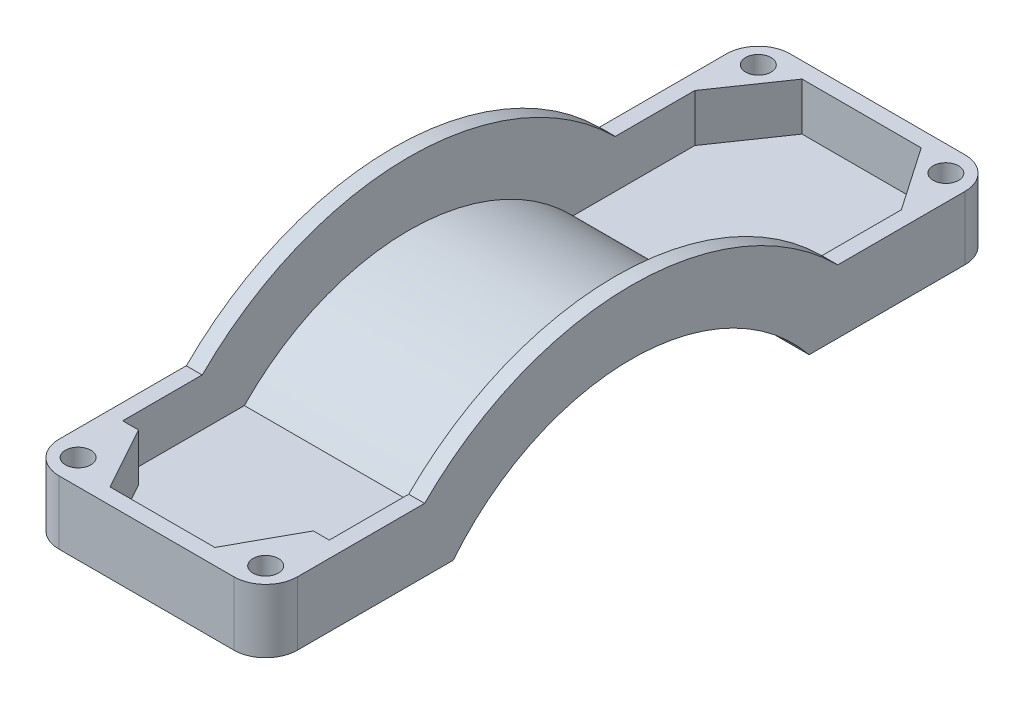
ISO-10303-21;
HEADER;
FILE_DESCRIPTION(('STEP AP214'),'2;1');
FILE_NAME('part.step','',(''),(''),'','','');
FILE_SCHEMA(('AUTOMOTIVE_DESIGN { 1 0 10303 214 1 1 1 1 }'));
ENDSEC;
DATA;
#1=APPLICATION_CONTEXT('core data for automotive mechanical design processes');
#2=APPLICATION_PROTOCOL_DEFINITION('international standard','automotive_design',2000,#1);
#3=PRODUCT_CONTEXT('',#1,'mechanical');
#4=PRODUCT('Part','Part','',(#3));
#5=PRODUCT_RELATED_PRODUCT_CATEGORY('part','',(#4));
#6=PRODUCT_DEFINITION_FORMATION('','',#4);
#7=PRODUCT_DEFINITION_CONTEXT('part definition',#1,'design');
#8=PRODUCT_DEFINITION('design','',#6,#7);
#9=PRODUCT_DEFINITION_SHAPE('','',#8);
#10=(LENGTH_UNIT() NAMED_UNIT(*) SI_UNIT(.MILLI.,.METRE.));
#11=(NAMED_UNIT(*) PLANE_ANGLE_UNIT() SI_UNIT($,.RADIAN.));
#12=(NAMED_UNIT(*) SI_UNIT($,.STERADIAN.) SOLID_ANGLE_UNIT());
#13=UNCERTAINTY_MEASURE_WITH_UNIT(LENGTH_MEASURE(1.E-05),#10,'distance_accuracy_value','');
#14=(GEOMETRIC_REPRESENTATION_CONTEXT(3) GLOBAL_UNCERTAINTY_ASSIGNED_CONTEXT((#13)) GLOBAL_UNIT_ASSIGNED_CONTEXT((#10,
#11,#12)) REPRESENTATION_CONTEXT('',''));
#15=CARTESIAN_POINT('',(0.,0.,0.));
#16=DIRECTION('',(0.,0.,1.));
#17=DIRECTION('',(1.,0.,0.));
#18=AXIS2_PLACEMENT_3D('',#15,#16,#17);
#19=CARTESIAN_POINT('',(-5.,0.,0.));
#20=DIRECTION('',(1.,0.,0.));
#21=DIRECTION('',(0.,0.,-1.));
#22=AXIS2_PLACEMENT_3D('',#19,#20,#21);
#23=PLANE('',#22);
#24=DIRECTION('',(0.,0.,-1.));
#25=VECTOR('',#24,1.);
#26=CARTESIAN_POINT('',(-5.00000000000001,50.1076032426321,0.));
#27=LINE('',#26,#25);
#28=CARTESIAN_POINT('',(-5.,50.1076032426321,-51.7032696962094));
#29=VERTEX_POINT('',#28);
#30=CARTESIAN_POINT('',(-5.,50.1076032426321,-90.));
#31=VERTEX_POINT('',#30);
#32=EDGE_CURVE('E569',#29,#31,#27,.T.);
#33=ORIENTED_EDGE('',*,*,#32,.F.);
#34=CARTESIAN_POINT('',(-5.,0.,0.));
#35=DIRECTION('',(1.,0.,0.));
#36=DIRECTION('',(0.,0.,-1.));
#37=AXIS2_PLACEMENT_3D('',#34,#35,#36);
#38=CIRCLE('',#37,72.);
#39=CARTESIAN_POINT('',(-5.,50.1076032426321,51.7032696962094));
#40=VERTEX_POINT('',#39);
#41=EDGE_CURVE('E249',#29,#40,#38,.T.);
#42=ORIENTED_EDGE('',*,*,#41,.T.);
#43=DIRECTION('',(0.,0.,1.));
#44=VECTOR('',#43,1.);
#45=CARTESIAN_POINT('',(-4.99999999999999,50.1076032426321,0.));
#46=LINE('',#45,#44);
#47=CARTESIAN_POINT('',(-5.,50.1076032426321,90.));
#48=VERTEX_POINT('',#47);
#49=EDGE_CURVE('E296',#40,#48,#46,.T.);
#50=ORIENTED_EDGE('',*,*,#49,.T.);
#51=DIRECTION('',(0.,1.,0.));
#52=VECTOR('',#51,1.);
#53=CARTESIAN_POINT('',(-5.,50.1076032426321,90.));
#54=LINE('',#53,#52);
#55=CARTESIAN_POINT('',(-5.,65.1076032426321,90.));
#56=VERTEX_POINT('',#55);
#57=EDGE_CURVE('E333',#48,#56,#54,.T.);
#58=ORIENTED_EDGE('',*,*,#57,.T.);
#59=DIRECTION('',(0.,0.,1.));
#60=VECTOR('',#59,1.);
#61=CARTESIAN_POINT('',(-4.99999999999999,65.1076032426321,0.));
#62=LINE('',#61,#60);
#63=CARTESIAN_POINT('',(-5.,65.1076032426321,65.));
#64=VERTEX_POINT('',#63);
#65=EDGE_CURVE('E317',#64,#56,#62,.T.);
#66=ORIENTED_EDGE('',*,*,#65,.F.);
#67=CARTESIAN_POINT('',(-5.,0.,0.));
#68=DIRECTION('',(1.,0.,0.));
#69=DIRECTION('',(0.,0.,-1.));
#70=AXIS2_PLACEMENT_3D('',#67,#68,#69);
#71=CIRCLE('',#70,92.);
#72=CARTESIAN_POINT('',(-5.,65.1076032426321,-65.));
#73=VERTEX_POINT('',#72);
#74=EDGE_CURVE('E348',#73,#64,#71,.T.);
#75=ORIENTED_EDGE('',*,*,#74,.F.);
#76=DIRECTION('',(0.,0.,-1.));
#77=VECTOR('',#76,1.);
#78=CARTESIAN_POINT('',(-5.00000000000001,65.1076032426321,0.));
#79=LINE('',#78,#77);
#80=CARTESIAN_POINT('',(-5.,65.1076032426321,-90.));
#81=VERTEX_POINT('',#80);
#82=EDGE_CURVE('E252',#73,#81,#79,.T.);
#83=ORIENTED_EDGE('',*,*,#82,.T.);
#84=DIRECTION('',(0.,1.,0.));
#85=VECTOR('',#84,1.);
#86=CARTESIAN_POINT('',(-5.,50.1076032426321,-90.));
#87=LINE('',#86,#85);
#88=EDGE_CURVE('E243',#31,#81,#87,.T.);
#89=ORIENTED_EDGE('',*,*,#88,.F.);
#90=EDGE_LOOP('',(#33,#42,#50,#58,#66,#75,#83,#89));
#91=FACE_BOUND('',#90,.T.);
#92=ADVANCED_FACE('F50',(#91),#23,.F.);
#93=CARTESIAN_POINT('',(-70.,50.1076032426321,0.));
#94=DIRECTION('',(1.,0.,0.));
#95=DIRECTION('',(0.,0.,-1.));
#96=AXIS2_PLACEMENT_3D('',#93,#94,#95);
#97=PLANE('',#96);
#98=CARTESIAN_POINT('',(-70.,0.,0.));
#99=DIRECTION('',(-1.,0.,0.));
#100=DIRECTION('',(0.,0.,1.));
#101=AXIS2_PLACEMENT_3D('',#98,#99,#100);
#102=CIRCLE('',#101,72.);
#103=CARTESIAN_POINT('',(-70.,50.1076032426321,51.7032696962094));
#104=VERTEX_POINT('',#103);
#105=CARTESIAN_POINT('',(-70.,50.1076032426321,-51.7032696962094));
#106=VERTEX_POINT('',#105);
#107=EDGE_CURVE('E248',#104,#106,#102,.T.);
#108=ORIENTED_EDGE('',*,*,#107,.T.);
#109=DIRECTION('',(0.,0.,1.));
#110=VECTOR('',#109,1.);
#111=CARTESIAN_POINT('',(-70.,50.1076032426321,0.));
#112=LINE('',#111,#110);
#113=CARTESIAN_POINT('',(-70.,50.1076032426321,-90.));
#114=VERTEX_POINT('',#113);
#115=EDGE_CURVE('E231',#114,#106,#112,.T.);
#116=ORIENTED_EDGE('',*,*,#115,.F.);
#117=DIRECTION('',(0.,1.,0.));
#118=VECTOR('',#117,1.);
#119=CARTESIAN_POINT('',(-70.,50.1076032426321,-90.));
#120=LINE('',#119,#118);
#121=CARTESIAN_POINT('',(-70.,65.1076032426321,-90.));
#122=VERTEX_POINT('',#121);
#123=EDGE_CURVE('E561',#114,#122,#120,.T.);
#124=ORIENTED_EDGE('',*,*,#123,.T.);
#125=DIRECTION('',(0.,0.,1.));
#126=VECTOR('',#125,1.);
#127=CARTESIAN_POINT('',(-70.,65.1076032426321,0.));
#128=LINE('',#127,#126);
#129=CARTESIAN_POINT('',(-70.,65.1076032426321,-65.));
#130=VERTEX_POINT('',#129);
#131=EDGE_CURVE('E568',#122,#130,#128,.T.);
#132=ORIENTED_EDGE('',*,*,#131,.T.);
#133=DIRECTION('',(0.,1.,0.));
#134=VECTOR('',#133,1.);
#135=CARTESIAN_POINT('',(-70.,0.,-65.));
#136=LINE('',#135,#134);
#137=CARTESIAN_POINT('',(-70.,65.0438347815245,-65.));
#138=VERTEX_POINT('',#137);
#139=EDGE_CURVE('E379',#138,#130,#136,.T.);
#140=ORIENTED_EDGE('',*,*,#139,.F.);
#141=CARTESIAN_POINT('',(-70.,0.,0.));
#142=DIRECTION('',(-1.,0.,0.));
#143=DIRECTION('',(0.,0.,1.));
#144=AXIS2_PLACEMENT_3D('',#141,#142,#143);
#145=CIRCLE('',#144,91.954882649516);
#146=CARTESIAN_POINT('',(-70.,65.0438347815245,65.));
#147=VERTEX_POINT('',#146);
#148=EDGE_CURVE('E257',#147,#138,#145,.T.);
#149=ORIENTED_EDGE('',*,*,#148,.F.);
#150=DIRECTION('',(0.,1.,0.));
#151=VECTOR('',#150,1.);
#152=CARTESIAN_POINT('',(-70.,50.1076032426321,65.));
#153=LINE('',#152,#151);
#154=CARTESIAN_POINT('',(-70.,65.1076032426321,65.));
#155=VERTEX_POINT('',#154);
#156=EDGE_CURVE('E326',#147,#155,#153,.T.);
#157=ORIENTED_EDGE('',*,*,#156,.T.);
#158=DIRECTION('',(0.,0.,-1.));
#159=VECTOR('',#158,1.);
#160=CARTESIAN_POINT('',(-70.,65.1076032426321,0.));
#161=LINE('',#160,#159);
#162=CARTESIAN_POINT('',(-70.,65.1076032426321,90.));
#163=VERTEX_POINT('',#162);
#164=EDGE_CURVE('E316',#163,#155,#161,.T.);
#165=ORIENTED_EDGE('',*,*,#164,.F.);
#166=DIRECTION('',(0.,1.,0.));
#167=VECTOR('',#166,1.);
#168=CARTESIAN_POINT('',(-70.,50.1076032426321,90.));
#169=LINE('',#168,#167);
#170=CARTESIAN_POINT('',(-70.,50.1076032426321,90.));
#171=VERTEX_POINT('',#170);
#172=EDGE_CURVE('E329',#171,#163,#169,.T.);
#173=ORIENTED_EDGE('',*,*,#172,.F.);
#174=DIRECTION('',(0.,0.,-1.));
#175=VECTOR('',#174,1.);
#176=CARTESIAN_POINT('',(-70.,50.1076032426321,0.));
#177=LINE('',#176,#175);
#178=EDGE_CURVE('E256',#171,#104,#177,.T.);
#179=ORIENTED_EDGE('',*,*,#178,.T.);
#180=EDGE_LOOP('',(#108,#116,#124,#132,#140,#149,#157,#165,#173,#179));
#181=FACE_BOUND('',#180,.T.);
#182=ADVANCED_FACE('F251',(#181),#97,.T.);
#183=CARTESIAN_POINT('',(-70.,0.,0.));
#184=DIRECTION('',(-1.,0.,0.));
#185=DIRECTION('',(0.,0.,1.));
#186=AXIS2_PLACEMENT_3D('',#183,#184,#185);
#187=CYLINDRICAL_SURFACE('',#186,91.954882649516);
#188=ORIENTED_EDGE('',*,*,#148,.T.);
#189=DIRECTION('',(-1.,0.,0.));
#190=VECTOR('',#189,1.);
#191=CARTESIAN_POINT('',(-70.,65.0438347815245,-65.));
#192=LINE('',#191,#190);
#193=CARTESIAN_POINT('',(-75.,65.0438347815245,-65.));
#194=VERTEX_POINT('',#193);
#195=EDGE_CURVE('E370',#138,#194,#192,.T.);
#196=ORIENTED_EDGE('',*,*,#195,.T.);
#197=CARTESIAN_POINT('',(-75.,0.,0.));
#198=DIRECTION('',(-1.,0.,0.));
#199=DIRECTION('',(0.,0.,1.));
#200=AXIS2_PLACEMENT_3D('',#197,#198,#199);
#201=CIRCLE('',#200,91.954882649516);
#202=CARTESIAN_POINT('',(-75.,65.0438347815245,65.));
#203=VERTEX_POINT('',#202);
#204=EDGE_CURVE('E258',#203,#194,#201,.T.);
#205=ORIENTED_EDGE('',*,*,#204,.F.);
#206=DIRECTION('',(-1.,0.,0.));
#207=VECTOR('',#206,1.);
#208=CARTESIAN_POINT('',(-70.,65.0438347815245,65.));
#209=LINE('',#208,#207);
#210=EDGE_CURVE('E264',#147,#203,#209,.T.);
#211=ORIENTED_EDGE('',*,*,#210,.F.);
#212=EDGE_LOOP('',(#188,#196,#205,#211));
#213=FACE_BOUND('',#212,.T.);
#214=ADVANCED_FACE('F459',(#213),#187,.T.);
#215=CARTESIAN_POINT('',(-75.,0.,0.));
#216=DIRECTION('',(1.,0.,0.));
#217=DIRECTION('',(0.,0.,-1.));
#218=AXIS2_PLACEMENT_3D('',#215,#216,#217);
#219=CYLINDRICAL_SURFACE('',#218,72.);
#220=DIRECTION('',(1.,0.,0.));
#221=VECTOR('',#220,1.);
#222=CARTESIAN_POINT('',(-75.,50.1076032426321,-51.7032696962094));
#223=LINE('',#222,#221);
#224=EDGE_CURVE('E240',#106,#29,#223,.T.);
#225=ORIENTED_EDGE('',*,*,#224,.F.);
#226=ORIENTED_EDGE('',*,*,#107,.F.);
#227=DIRECTION('',(1.,0.,0.));
#228=VECTOR('',#227,1.);
#229=CARTESIAN_POINT('',(-75.,50.1076032426321,51.7032696962094));
#230=LINE('',#229,#228);
#231=EDGE_CURVE('E263',#40,#104,#230,.F.);
#232=ORIENTED_EDGE('',*,*,#231,.F.);
#233=ORIENTED_EDGE('',*,*,#41,.F.);
#234=EDGE_LOOP('',(#225,#226,#232,#233));
#235=FACE_BOUND('',#234,.T.);
#236=ADVANCED_FACE('F250',(#235),#219,.T.);
#237=CARTESIAN_POINT('',(-5.,65.1076032426321,0.));
#238=DIRECTION('',(0.,1.,0.));
#239=DIRECTION('',(0.,0.,1.));
#240=AXIS2_PLACEMENT_3D('',#237,#238,#239);
#241=PLANE('',#240);
#242=CARTESIAN_POINT('',(-8.,65.1076032426321,107.));
#243=DIRECTION('',(0.,1.,0.));
#244=DIRECTION('',(0.,0.,1.));
#245=AXIS2_PLACEMENT_3D('',#242,#243,#244);
#246=CIRCLE('',#245,4.);
#247=CARTESIAN_POINT('',(-8.,65.1076032426321,111.));
#248=VERTEX_POINT('',#247);
#249=EDGE_CURVE('E593',#248,#248,#246,.T.);
#250=ORIENTED_EDGE('',*,*,#249,.F.);
#251=EDGE_LOOP('',(#250));
#252=FACE_BOUND('',#251,.T.);
#253=CARTESIAN_POINT('',(-67.,65.1076032426321,107.));
#254=DIRECTION('',(0.,1.,0.));
#255=DIRECTION('',(0.,0.,1.));
#256=AXIS2_PLACEMENT_3D('',#253,#254,#255);
#257=CIRCLE('',#256,4.00000000000001);
#258=CARTESIAN_POINT('',(-67.,65.1076032426321,111.));
#259=VERTEX_POINT('',#258);
#260=EDGE_CURVE('E595',#259,#259,#257,.T.);
#261=ORIENTED_EDGE('',*,*,#260,.F.);
#262=EDGE_LOOP('',(#261));
#263=FACE_BOUND('',#262,.T.);
#264=DIRECTION('',(0.,0.,1.));
#265=VECTOR('',#264,1.);
#266=CARTESIAN_POINT('',(-75.,65.1076032426321,65.));
#267=LINE('',#266,#265);
#268=CARTESIAN_POINT('',(-75.,65.1076032426321,65.));
#269=VERTEX_POINT('',#268);
#270=CARTESIAN_POINT('',(-75.,65.1076032426321,105.));
#271=VERTEX_POINT('',#270);
#272=EDGE_CURVE('E345',#269,#271,#267,.T.);
#273=ORIENTED_EDGE('',*,*,#272,.T.);
#274=CARTESIAN_POINT('',(-65.,65.1076032426321,105.));
#275=DIRECTION('',(0.,1.,0.));
#276=DIRECTION('',(0.,0.,1.));
#277=AXIS2_PLACEMENT_3D('',#274,#275,#276);
#278=CIRCLE('',#277,10.);
#279=CARTESIAN_POINT('',(-65.,65.1076032426321,115.));
#280=VERTEX_POINT('',#279);
#281=EDGE_CURVE('E415',#271,#280,#278,.T.);
#282=ORIENTED_EDGE('',*,*,#281,.T.);
#283=DIRECTION('',(1.,0.,0.));
#284=VECTOR('',#283,1.);
#285=CARTESIAN_POINT('',(-5.,65.1076032426321,115.));
#286=LINE('',#285,#284);
#287=CARTESIAN_POINT('',(-10.,65.1076032426321,115.));
#288=VERTEX_POINT('',#287);
#289=EDGE_CURVE('E368',#280,#288,#286,.T.);
#290=ORIENTED_EDGE('',*,*,#289,.T.);
#291=CARTESIAN_POINT('',(-10.,65.1076032426321,105.));
#292=DIRECTION('',(0.,1.,0.));
#293=DIRECTION('',(0.,0.,1.));
#294=AXIS2_PLACEMENT_3D('',#291,#292,#293);
#295=CIRCLE('',#294,10.);
#296=CARTESIAN_POINT('',(0.,65.1076032426321,105.));
#297=VERTEX_POINT('',#296);
#298=EDGE_CURVE('E404',#288,#297,#295,.T.);
#299=ORIENTED_EDGE('',*,*,#298,.T.);
#300=DIRECTION('',(0.,0.,1.));
#301=VECTOR('',#300,1.);
#302=CARTESIAN_POINT('',(0.,65.1076032426321,0.));
#303=LINE('',#302,#301);
#304=CARTESIAN_POINT('',(0.,65.1076032426321,65.));
#305=VERTEX_POINT('',#304);
#306=EDGE_CURVE('E363',#305,#297,#303,.T.);
#307=ORIENTED_EDGE('',*,*,#306,.F.);
#308=DIRECTION('',(1.,0.,0.));
#309=VECTOR('',#308,1.);
#310=CARTESIAN_POINT('',(-5.,65.1076032426321,65.));
#311=LINE('',#310,#309);
#312=EDGE_CURVE('E369',#64,#305,#311,.T.);
#313=ORIENTED_EDGE('',*,*,#312,.F.);
#314=ORIENTED_EDGE('',*,*,#65,.T.);
#315=DIRECTION('',(-1.,0.,0.));
#316=VECTOR('',#315,1.);
#317=CARTESIAN_POINT('',(0.,65.1076032426321,90.));
#318=LINE('',#317,#316);
#319=CARTESIAN_POINT('',(-10.,65.1076032426321,90.));
#320=VERTEX_POINT('',#319);
#321=EDGE_CURVE('E312',#56,#320,#318,.T.);
#322=ORIENTED_EDGE('',*,*,#321,.T.);
#323=DIRECTION('',(0.481918749772156,0.,-0.876215908676647));
#324=VECTOR('',#323,1.);
#325=CARTESIAN_POINT('',(30.3262955854127,65.1076032426321,16.679462571977));
#326=LINE('',#325,#324);
#327=CARTESIAN_POINT('',(-21.,65.1076032426321,110.));
#328=VERTEX_POINT('',#327);
#329=EDGE_CURVE('E309',#328,#320,#326,.T.);
#330=ORIENTED_EDGE('',*,*,#329,.F.);
#331=DIRECTION('',(1.,0.,0.));
#332=VECTOR('',#331,1.);
#333=CARTESIAN_POINT('',(0.,65.1076032426321,110.));
#334=LINE('',#333,#332);
#335=CARTESIAN_POINT('',(-54.,65.1076032426321,110.));
#336=VERTEX_POINT('',#335);
#337=EDGE_CURVE('E310',#336,#328,#334,.T.);
#338=ORIENTED_EDGE('',*,*,#337,.F.);
#339=DIRECTION('',(0.481918749772156,0.,0.876215908676647));
#340=VECTOR('',#339,1.);
#341=CARTESIAN_POINT('',(-87.9078694817658,65.1076032426321,48.3493282149712));
#342=LINE('',#341,#340);
#343=CARTESIAN_POINT('',(-65.,65.1076032426321,90.));
#344=VERTEX_POINT('',#343);
#345=EDGE_CURVE('E285',#344,#336,#342,.T.);
#346=ORIENTED_EDGE('',*,*,#345,.F.);
#347=DIRECTION('',(1.,0.,0.));
#348=VECTOR('',#347,1.);
#349=CARTESIAN_POINT('',(0.,65.1076032426321,90.));
#350=LINE('',#349,#348);
#351=EDGE_CURVE('E286',#163,#344,#350,.T.);
#352=ORIENTED_EDGE('',*,*,#351,.F.);
#353=ORIENTED_EDGE('',*,*,#164,.T.);
#354=DIRECTION('',(-1.,0.,0.));
#355=VECTOR('',#354,1.);
#356=CARTESIAN_POINT('',(-5.,65.1076032426321,65.));
#357=LINE('',#356,#355);
#358=EDGE_CURVE('E327',#155,#269,#357,.T.);
#359=ORIENTED_EDGE('',*,*,#358,.T.);
#360=EDGE_LOOP('',(#273,#282,#290,#299,#307,#313,#314,#322,#330,#338,#346,#352,#353,#359));
#361=FACE_BOUND('',#360,.T.);
#362=ADVANCED_FACE('F477',(#252,#263,#361),#241,.T.);
#363=CARTESIAN_POINT('',(0.,0.,65.));
#364=DIRECTION('',(0.,0.,-1.));
#365=DIRECTION('',(-1.,0.,0.));
#366=AXIS2_PLACEMENT_3D('',#363,#364,#365);
#367=PLANE('',#366);
#368=ORIENTED_EDGE('',*,*,#210,.T.);
#369=DIRECTION('',(0.,-1.,0.));
#370=VECTOR('',#369,1.);
#371=CARTESIAN_POINT('',(-75.,45.1076032426321,65.));
#372=LINE('',#371,#370);
#373=EDGE_CURVE('E339',#269,#203,#372,.T.);
#374=ORIENTED_EDGE('',*,*,#373,.F.);
#375=ORIENTED_EDGE('',*,*,#358,.F.);
#376=ORIENTED_EDGE('',*,*,#156,.F.);
#377=EDGE_LOOP('',(#368,#374,#375,#376));
#378=FACE_BOUND('',#377,.T.);
#379=ADVANCED_FACE('F468',(#378),#367,.T.);
#380=CARTESIAN_POINT('',(-5.,45.1076032426321,0.));
#381=DIRECTION('',(0.,-1.,0.));
#382=DIRECTION('',(0.,0.,-1.));
#383=AXIS2_PLACEMENT_3D('',#380,#381,#382);
#384=PLANE('',#383);
#385=CARTESIAN_POINT('',(-8.,45.1076032426321,107.));
#386=DIRECTION('',(0.,-1.,0.));
#387=DIRECTION('',(0.,0.,-1.));
#388=AXIS2_PLACEMENT_3D('',#385,#386,#387);
#389=CIRCLE('',#388,4.);
#390=CARTESIAN_POINT('',(-8.,45.1076032426321,103.));
#391=VERTEX_POINT('',#390);
#392=EDGE_CURVE('E255',#391,#391,#389,.T.);
#393=ORIENTED_EDGE('',*,*,#392,.F.);
#394=EDGE_LOOP('',(#393));
#395=FACE_BOUND('',#394,.T.);
#396=CARTESIAN_POINT('',(-67.,45.1076032426321,107.));
#397=DIRECTION('',(0.,-1.,0.));
#398=DIRECTION('',(0.,0.,-1.));
#399=AXIS2_PLACEMENT_3D('',#396,#397,#398);
#400=CIRCLE('',#399,4.00000000000001);
#401=CARTESIAN_POINT('',(-67.,45.1076032426321,103.));
#402=VERTEX_POINT('',#401);
#403=EDGE_CURVE('E392',#402,#402,#400,.T.);
#404=ORIENTED_EDGE('',*,*,#403,.F.);
#405=EDGE_LOOP('',(#404));
#406=FACE_BOUND('',#405,.T.);
#407=DIRECTION('',(1.,0.,0.));
#408=VECTOR('',#407,1.);
#409=CARTESIAN_POINT('',(-5.,45.1076032426321,115.));
#410=LINE('',#409,#408);
#411=CARTESIAN_POINT('',(-65.,45.1076032426321,115.));
#412=VERTEX_POINT('',#411);
#413=CARTESIAN_POINT('',(-10.,45.1076032426321,115.));
#414=VERTEX_POINT('',#413);
#415=EDGE_CURVE('E362',#412,#414,#410,.T.);
#416=ORIENTED_EDGE('',*,*,#415,.F.);
#417=CARTESIAN_POINT('',(-65.,45.1076032426321,105.));
#418=DIRECTION('',(0.,-1.,0.));
#419=DIRECTION('',(0.,0.,-1.));
#420=AXIS2_PLACEMENT_3D('',#417,#418,#419);
#421=CIRCLE('',#420,10.);
#422=CARTESIAN_POINT('',(-75.,45.1076032426321,105.));
#423=VERTEX_POINT('',#422);
#424=EDGE_CURVE('E408',#412,#423,#421,.T.);
#425=ORIENTED_EDGE('',*,*,#424,.T.);
#426=DIRECTION('',(0.,0.,1.));
#427=VECTOR('',#426,1.);
#428=CARTESIAN_POINT('',(-75.,45.1076032426321,65.));
#429=LINE('',#428,#427);
#430=CARTESIAN_POINT('',(-75.,45.1076032426321,55.9862114949478));
#431=VERTEX_POINT('',#430);
#432=EDGE_CURVE('E342',#431,#423,#429,.T.);
#433=ORIENTED_EDGE('',*,*,#432,.F.);
#434=DIRECTION('',(1.,0.,0.));
#435=VECTOR('',#434,1.);
#436=CARTESIAN_POINT('',(-75.,45.1076032426321,55.9862114949478));
#437=LINE('',#436,#435);
#438=CARTESIAN_POINT('',(0.,45.1076032426321,55.9862114949478));
#439=VERTEX_POINT('',#438);
#440=EDGE_CURVE('E277',#431,#439,#437,.T.);
#441=ORIENTED_EDGE('',*,*,#440,.T.);
#442=DIRECTION('',(0.,0.,-1.));
#443=VECTOR('',#442,1.);
#444=CARTESIAN_POINT('',(0.,45.1076032426321,0.));
#445=LINE('',#444,#443);
#446=CARTESIAN_POINT('',(0.,45.1076032426321,105.));
#447=VERTEX_POINT('',#446);
#448=EDGE_CURVE('E353',#447,#439,#445,.T.);
#449=ORIENTED_EDGE('',*,*,#448,.F.);
#450=CARTESIAN_POINT('',(-10.,45.1076032426321,105.));
#451=DIRECTION('',(0.,-1.,0.));
#452=DIRECTION('',(0.,0.,-1.));
#453=AXIS2_PLACEMENT_3D('',#450,#451,#452);
#454=CIRCLE('',#453,10.);
#455=EDGE_CURVE('E397',#447,#414,#454,.T.);
#456=ORIENTED_EDGE('',*,*,#455,.T.);
#457=EDGE_LOOP('',(#416,#425,#433,#441,#449,#456));
#458=FACE_BOUND('',#457,.T.);
#459=ADVANCED_FACE('F467',(#395,#406,#458),#384,.T.);
#460=CARTESIAN_POINT('',(-5.,0.,115.));
#461=DIRECTION('',(0.,0.,1.));
#462=DIRECTION('',(1.,0.,0.));
#463=AXIS2_PLACEMENT_3D('',#460,#461,#462);
#464=PLANE('',#463);
#465=ORIENTED_EDGE('',*,*,#289,.F.);
#466=DIRECTION('',(0.,-1.,0.));
#467=VECTOR('',#466,1.);
#468=CARTESIAN_POINT('',(-65.,0.,115.));
#469=LINE('',#468,#467);
#470=EDGE_CURVE('E406',#280,#412,#469,.T.);
#471=ORIENTED_EDGE('',*,*,#470,.T.);
#472=ORIENTED_EDGE('',*,*,#415,.T.);
#473=DIRECTION('',(0.,-1.,0.));
#474=VECTOR('',#473,1.);
#475=CARTESIAN_POINT('',(-10.,0.,115.));
#476=LINE('',#475,#474);
#477=EDGE_CURVE('E402',#414,#288,#476,.F.);
#478=ORIENTED_EDGE('',*,*,#477,.T.);
#479=EDGE_LOOP('',(#465,#471,#472,#478));
#480=FACE_BOUND('',#479,.T.);
#481=ADVANCED_FACE('F469',(#480),#464,.T.);
#482=CARTESIAN_POINT('',(-5.,0.,0.));
#483=DIRECTION('',(1.,0.,0.));
#484=DIRECTION('',(0.,0.,-1.));
#485=AXIS2_PLACEMENT_3D('',#482,#483,#484);
#486=CYLINDRICAL_SURFACE('',#485,92.);
#487=CARTESIAN_POINT('',(0.,0.,0.));
#488=DIRECTION('',(1.,0.,0.));
#489=DIRECTION('',(0.,0.,-1.));
#490=AXIS2_PLACEMENT_3D('',#487,#488,#489);
#491=CIRCLE('',#490,92.);
#492=CARTESIAN_POINT('',(0.,65.1076032426321,-65.));
#493=VERTEX_POINT('',#492);
#494=EDGE_CURVE('E356',#493,#305,#491,.T.);
#495=ORIENTED_EDGE('',*,*,#494,.F.);
#496=DIRECTION('',(1.,0.,0.));
#497=VECTOR('',#496,1.);
#498=CARTESIAN_POINT('',(-5.,65.1076032426321,-65.));
#499=LINE('',#498,#497);
#500=EDGE_CURVE('E375',#73,#493,#499,.T.);
#501=ORIENTED_EDGE('',*,*,#500,.F.);
#502=ORIENTED_EDGE('',*,*,#74,.T.);
#503=ORIENTED_EDGE('',*,*,#312,.T.);
#504=EDGE_LOOP('',(#495,#501,#502,#503));
#505=FACE_BOUND('',#504,.T.);
#506=ADVANCED_FACE('F473',(#505),#486,.T.);
#507=CARTESIAN_POINT('',(-5.,65.1076032426321,0.));
#508=DIRECTION('',(0.,-1.,0.));
#509=DIRECTION('',(0.,0.,-1.));
#510=AXIS2_PLACEMENT_3D('',#507,#508,#509);
#511=PLANE('',#510);
#512=CARTESIAN_POINT('',(-67.,65.1076032426321,-107.));
#513=DIRECTION('',(0.,1.,0.));
#514=DIRECTION('',(0.,0.,1.));
#515=AXIS2_PLACEMENT_3D('',#512,#513,#514);
#516=CIRCLE('',#515,4.00000000000001);
#517=CARTESIAN_POINT('',(-67.,65.1076032426321,-103.));
#518=VERTEX_POINT('',#517);
#519=EDGE_CURVE('E588',#518,#518,#516,.T.);
#520=ORIENTED_EDGE('',*,*,#519,.F.);
#521=EDGE_LOOP('',(#520));
#522=FACE_BOUND('',#521,.T.);
#523=CARTESIAN_POINT('',(-8.,65.1076032426321,-107.));
#524=DIRECTION('',(0.,1.,0.));
#525=DIRECTION('',(0.,0.,1.));
#526=AXIS2_PLACEMENT_3D('',#523,#524,#525);
#527=CIRCLE('',#526,4.);
#528=CARTESIAN_POINT('',(-8.,65.1076032426321,-103.));
#529=VERTEX_POINT('',#528);
#530=EDGE_CURVE('E387',#529,#529,#527,.T.);
#531=ORIENTED_EDGE('',*,*,#530,.F.);
#532=EDGE_LOOP('',(#531));
#533=FACE_BOUND('',#532,.T.);
#534=DIRECTION('',(0.,0.,-1.));
#535=VECTOR('',#534,1.);
#536=CARTESIAN_POINT('',(0.,65.1076032426321,0.));
#537=LINE('',#536,#535);
#538=CARTESIAN_POINT('',(0.,65.1076032426321,-105.));
#539=VERTEX_POINT('',#538);
#540=EDGE_CURVE('E358',#493,#539,#537,.T.);
#541=ORIENTED_EDGE('',*,*,#540,.T.);
#542=CARTESIAN_POINT('',(-10.,65.1076032426321,-105.));
#543=DIRECTION('',(0.,-1.,0.));
#544=DIRECTION('',(0.,0.,-1.));
#545=AXIS2_PLACEMENT_3D('',#542,#543,#544);
#546=CIRCLE('',#545,10.);
#547=CARTESIAN_POINT('',(-10.,65.1076032426321,-115.));
#548=VERTEX_POINT('',#547);
#549=EDGE_CURVE('E11',#539,#548,#546,.F.);
#550=ORIENTED_EDGE('',*,*,#549,.T.);
#551=DIRECTION('',(1.,0.,0.));
#552=VECTOR('',#551,1.);
#553=CARTESIAN_POINT('',(-5.,65.1076032426321,-115.));
#554=LINE('',#553,#552);
#555=CARTESIAN_POINT('',(-65.,65.1076032426321,-115.));
#556=VERTEX_POINT('',#555);
#557=EDGE_CURVE('E372',#556,#548,#554,.T.);
#558=ORIENTED_EDGE('',*,*,#557,.F.);
#559=CARTESIAN_POINT('',(-65.,65.1076032426321,-105.));
#560=DIRECTION('',(0.,-1.,0.));
#561=DIRECTION('',(0.,0.,-1.));
#562=AXIS2_PLACEMENT_3D('',#559,#560,#561);
#563=CIRCLE('',#562,10.);
#564=CARTESIAN_POINT('',(-75.,65.1076032426321,-105.));
#565=VERTEX_POINT('',#564);
#566=EDGE_CURVE('E417',#556,#565,#563,.F.);
#567=ORIENTED_EDGE('',*,*,#566,.T.);
#568=DIRECTION('',(0.,0.,-1.));
#569=VECTOR('',#568,1.);
#570=CARTESIAN_POINT('',(-75.,65.1076032426321,-65.));
#571=LINE('',#570,#569);
#572=CARTESIAN_POINT('',(-75.,65.1076032426321,-65.));
#573=VERTEX_POINT('',#572);
#574=EDGE_CURVE('E551',#573,#565,#571,.T.);
#575=ORIENTED_EDGE('',*,*,#574,.F.);
#576=DIRECTION('',(1.,0.,0.));
#577=VECTOR('',#576,1.);
#578=CARTESIAN_POINT('',(-75.,65.1076032426321,-65.));
#579=LINE('',#578,#577);
#580=EDGE_CURVE('E560',#573,#130,#579,.T.);
#581=ORIENTED_EDGE('',*,*,#580,.T.);
#582=ORIENTED_EDGE('',*,*,#131,.F.);
#583=DIRECTION('',(0.566528822887065,0.,-0.824041924199368));
#584=VECTOR('',#583,1.);
#585=CARTESIAN_POINT('',(-89.5490716180371,65.1076032426321,-61.5649867374005));
#586=LINE('',#585,#584);
#587=CARTESIAN_POINT('',(-56.25,65.1076032426321,-110.));
#588=VERTEX_POINT('',#587);
#589=EDGE_CURVE('E571',#122,#588,#586,.T.);
#590=ORIENTED_EDGE('',*,*,#589,.T.);
#591=DIRECTION('',(1.,0.,0.));
#592=VECTOR('',#591,1.);
#593=CARTESIAN_POINT('',(0.,65.1076032426321,-110.));
#594=LINE('',#593,#592);
#595=CARTESIAN_POINT('',(-18.75,65.1076032426321,-110.));
#596=VERTEX_POINT('',#595);
#597=EDGE_CURVE('E573',#588,#596,#594,.T.);
#598=ORIENTED_EDGE('',*,*,#597,.T.);
#599=DIRECTION('',(-0.566528822887065,0.,-0.824041924199368));
#600=VECTOR('',#599,1.);
#601=CARTESIAN_POINT('',(38.6206896551724,65.1076032426321,-26.551724137931));
#602=LINE('',#601,#600);
#603=EDGE_CURVE('E580',#81,#596,#602,.T.);
#604=ORIENTED_EDGE('',*,*,#603,.F.);
#605=ORIENTED_EDGE('',*,*,#82,.F.);
#606=ORIENTED_EDGE('',*,*,#500,.T.);
#607=EDGE_LOOP('',(#541,#550,#558,#567,#575,#581,#582,#590,#598,#604,#605,#606));
#608=FACE_BOUND('',#607,.T.);
#609=ADVANCED_FACE('F442',(#522,#533,#608),#511,.F.);
#610=CARTESIAN_POINT('',(-5.,0.,-115.));
#611=DIRECTION('',(0.,0.,1.));
#612=DIRECTION('',(1.,0.,0.));
#613=AXIS2_PLACEMENT_3D('',#610,#611,#612);
#614=PLANE('',#613);
#615=ORIENTED_EDGE('',*,*,#557,.T.);
#616=DIRECTION('',(0.,-1.,0.));
#617=VECTOR('',#616,1.);
#618=CARTESIAN_POINT('',(-10.,45.1076032426321,-115.));
#619=LINE('',#618,#617);
#620=CARTESIAN_POINT('',(-10.,45.1076032426321,-115.));
#621=VERTEX_POINT('',#620);
#622=EDGE_CURVE('E425',#548,#621,#619,.T.);
#623=ORIENTED_EDGE('',*,*,#622,.T.);
#624=DIRECTION('',(1.,0.,0.));
#625=VECTOR('',#624,1.);
#626=CARTESIAN_POINT('',(-5.,45.1076032426321,-115.));
#627=LINE('',#626,#625);
#628=CARTESIAN_POINT('',(-65.,45.1076032426321,-115.));
#629=VERTEX_POINT('',#628);
#630=EDGE_CURVE('E355',#629,#621,#627,.T.);
#631=ORIENTED_EDGE('',*,*,#630,.F.);
#632=DIRECTION('',(0.,1.,0.));
#633=VECTOR('',#632,1.);
#634=CARTESIAN_POINT('',(-65.,65.1076032426321,-115.));
#635=LINE('',#634,#633);
#636=EDGE_CURVE('E413',#629,#556,#635,.T.);
#637=ORIENTED_EDGE('',*,*,#636,.T.);
#638=EDGE_LOOP('',(#615,#623,#631,#637));
#639=FACE_BOUND('',#638,.T.);
#640=ADVANCED_FACE('F427',(#639),#614,.F.);
#641=CARTESIAN_POINT('',(-5.,45.1076032426321,0.));
#642=DIRECTION('',(0.,-1.,0.));
#643=DIRECTION('',(0.,0.,-1.));
#644=AXIS2_PLACEMENT_3D('',#641,#642,#643);
#645=PLANE('',#644);
#646=CARTESIAN_POINT('',(-67.,45.1076032426321,-107.));
#647=DIRECTION('',(0.,-1.,0.));
#648=DIRECTION('',(0.,0.,-1.));
#649=AXIS2_PLACEMENT_3D('',#646,#647,#648);
#650=CIRCLE('',#649,4.00000000000001);
#651=CARTESIAN_POINT('',(-67.,45.1076032426321,-111.));
#652=VERTEX_POINT('',#651);
#653=EDGE_CURVE('E390',#652,#652,#650,.T.);
#654=ORIENTED_EDGE('',*,*,#653,.F.);
#655=EDGE_LOOP('',(#654));
#656=FACE_BOUND('',#655,.T.);
#657=CARTESIAN_POINT('',(-8.,45.1076032426321,-107.));
#658=DIRECTION('',(0.,-1.,0.));
#659=DIRECTION('',(0.,0.,-1.));
#660=AXIS2_PLACEMENT_3D('',#657,#658,#659);
#661=CIRCLE('',#660,4.);
#662=CARTESIAN_POINT('',(-8.,45.1076032426321,-111.));
#663=VERTEX_POINT('',#662);
#664=EDGE_CURVE('E381',#663,#663,#661,.T.);
#665=ORIENTED_EDGE('',*,*,#664,.F.);
#666=EDGE_LOOP('',(#665));
#667=FACE_BOUND('',#666,.T.);
#668=ORIENTED_EDGE('',*,*,#630,.T.);
#669=CARTESIAN_POINT('',(-10.,45.1076032426321,-105.));
#670=DIRECTION('',(0.,-1.,0.));
#671=DIRECTION('',(0.,0.,-1.));
#672=AXIS2_PLACEMENT_3D('',#669,#670,#671);
#673=CIRCLE('',#672,10.);
#674=CARTESIAN_POINT('',(0.,45.1076032426321,-105.));
#675=VERTEX_POINT('',#674);
#676=EDGE_CURVE('E66',#621,#675,#673,.T.);
#677=ORIENTED_EDGE('',*,*,#676,.T.);
#678=DIRECTION('',(0.,0.,-1.));
#679=VECTOR('',#678,1.);
#680=CARTESIAN_POINT('',(0.,45.1076032426321,0.));
#681=LINE('',#680,#679);
#682=CARTESIAN_POINT('',(0.,45.1076032426321,-55.9862114949478));
#683=VERTEX_POINT('',#682);
#684=EDGE_CURVE('E347',#683,#675,#681,.T.);
#685=ORIENTED_EDGE('',*,*,#684,.F.);
#686=DIRECTION('',(1.,0.,0.));
#687=VECTOR('',#686,1.);
#688=CARTESIAN_POINT('',(-75.,45.1076032426321,-55.9862114949478));
#689=LINE('',#688,#687);
#690=CARTESIAN_POINT('',(-75.,45.1076032426321,-55.9862114949478));
#691=VERTEX_POINT('',#690);
#692=EDGE_CURVE('E279',#691,#683,#689,.T.);
#693=ORIENTED_EDGE('',*,*,#692,.F.);
#694=DIRECTION('',(0.,0.,-1.));
#695=VECTOR('',#694,1.);
#696=CARTESIAN_POINT('',(-75.,45.1076032426321,-55.9862114949478));
#697=LINE('',#696,#695);
#698=CARTESIAN_POINT('',(-75.,45.1076032426321,-105.));
#699=VERTEX_POINT('',#698);
#700=EDGE_CURVE('E273',#691,#699,#697,.T.);
#701=ORIENTED_EDGE('',*,*,#700,.T.);
#702=CARTESIAN_POINT('',(-65.,45.1076032426321,-105.));
#703=DIRECTION('',(0.,-1.,0.));
#704=DIRECTION('',(0.,0.,-1.));
#705=AXIS2_PLACEMENT_3D('',#702,#703,#704);
#706=CIRCLE('',#705,10.);
#707=EDGE_CURVE('E422',#699,#629,#706,.T.);
#708=ORIENTED_EDGE('',*,*,#707,.T.);
#709=EDGE_LOOP('',(#668,#677,#685,#693,#701,#708));
#710=FACE_BOUND('',#709,.T.);
#711=ADVANCED_FACE('F434',(#656,#667,#710),#645,.T.);
#712=CARTESIAN_POINT('',(0.,0.,0.));
#713=DIRECTION('',(1.,0.,0.));
#714=DIRECTION('',(0.,0.,-1.));
#715=AXIS2_PLACEMENT_3D('',#712,#713,#714);
#716=PLANE('',#715);
#717=ORIENTED_EDGE('',*,*,#684,.T.);
#718=DIRECTION('',(0.,-1.,0.));
#719=VECTOR('',#718,1.);
#720=CARTESIAN_POINT('',(0.,65.1076032426321,-105.));
#721=LINE('',#720,#719);
#722=EDGE_CURVE('E54',#675,#539,#721,.F.);
#723=ORIENTED_EDGE('',*,*,#722,.T.);
#724=ORIENTED_EDGE('',*,*,#540,.F.);
#725=ORIENTED_EDGE('',*,*,#494,.T.);
#726=ORIENTED_EDGE('',*,*,#306,.T.);
#727=DIRECTION('',(0.,-1.,0.));
#728=VECTOR('',#727,1.);
#729=CARTESIAN_POINT('',(0.,0.,105.));
#730=LINE('',#729,#728);
#731=EDGE_CURVE('E384',#297,#447,#730,.T.);
#732=ORIENTED_EDGE('',*,*,#731,.T.);
#733=ORIENTED_EDGE('',*,*,#448,.T.);
#734=CARTESIAN_POINT('',(0.,0.,0.));
#735=DIRECTION('',(-1.,0.,0.));
#736=DIRECTION('',(0.,0.,-1.));
#737=AXIS2_PLACEMENT_3D('',#734,#735,#736);
#738=CIRCLE('',#737,71.8968131967734);
#739=EDGE_CURVE('E275',#439,#683,#738,.T.);
#740=ORIENTED_EDGE('',*,*,#739,.T.);
#741=EDGE_LOOP('',(#717,#723,#724,#725,#726,#732,#733,#740));
#742=FACE_BOUND('',#741,.T.);
#743=ADVANCED_FACE('F462',(#742),#716,.T.);
#744=CARTESIAN_POINT('',(-75.,45.1076032426321,65.));
#745=DIRECTION('',(-1.,0.,0.));
#746=DIRECTION('',(0.,0.,1.));
#747=AXIS2_PLACEMENT_3D('',#744,#745,#746);
#748=PLANE('',#747);
#749=ORIENTED_EDGE('',*,*,#574,.T.);
#750=DIRECTION('',(0.,1.,0.));
#751=VECTOR('',#750,1.);
#752=CARTESIAN_POINT('',(-75.,45.1076032426321,-105.));
#753=LINE('',#752,#751);
#754=EDGE_CURVE('E416',#565,#699,#753,.F.);
#755=ORIENTED_EDGE('',*,*,#754,.T.);
#756=ORIENTED_EDGE('',*,*,#700,.F.);
#757=CARTESIAN_POINT('',(-75.,0.,0.));
#758=DIRECTION('',(-1.,0.,0.));
#759=DIRECTION('',(0.,0.,-1.));
#760=AXIS2_PLACEMENT_3D('',#757,#758,#759);
#761=CIRCLE('',#760,71.8968131967734);
#762=EDGE_CURVE('E271',#431,#691,#761,.T.);
#763=ORIENTED_EDGE('',*,*,#762,.F.);
#764=ORIENTED_EDGE('',*,*,#432,.T.);
#765=DIRECTION('',(0.,-1.,0.));
#766=VECTOR('',#765,1.);
#767=CARTESIAN_POINT('',(-75.,45.1076032426321,105.));
#768=LINE('',#767,#766);
#769=EDGE_CURVE('E412',#423,#271,#768,.F.);
#770=ORIENTED_EDGE('',*,*,#769,.T.);
#771=ORIENTED_EDGE('',*,*,#272,.F.);
#772=ORIENTED_EDGE('',*,*,#373,.T.);
#773=ORIENTED_EDGE('',*,*,#204,.T.);
#774=DIRECTION('',(0.,1.,0.));
#775=VECTOR('',#774,1.);
#776=CARTESIAN_POINT('',(-75.,45.1076032426321,-65.));
#777=LINE('',#776,#775);
#778=EDGE_CURVE('E555',#194,#573,#777,.T.);
#779=ORIENTED_EDGE('',*,*,#778,.T.);
#780=EDGE_LOOP('',(#749,#755,#756,#763,#764,#770,#771,#772,#773,#779));
#781=FACE_BOUND('',#780,.T.);
#782=ADVANCED_FACE('F463',(#781),#748,.T.);
#783=CARTESIAN_POINT('',(-87.9078694817658,50.1076032426321,48.3493282149712));
#784=DIRECTION('',(-0.876215908676647,0.,0.481918749772156));
#785=DIRECTION('',(0.481918749772156,0.,0.876215908676647));
#786=AXIS2_PLACEMENT_3D('',#783,#784,#785);
#787=PLANE('',#786);
#788=ORIENTED_EDGE('',*,*,#345,.T.);
#789=DIRECTION('',(0.,1.,0.));
#790=VECTOR('',#789,1.);
#791=CARTESIAN_POINT('',(-54.,50.1076032426321,110.));
#792=LINE('',#791,#790);
#793=CARTESIAN_POINT('',(-54.,50.1076032426321,110.));
#794=VERTEX_POINT('',#793);
#795=EDGE_CURVE('E302',#794,#336,#792,.T.);
#796=ORIENTED_EDGE('',*,*,#795,.F.);
#797=DIRECTION('',(0.481918749772156,0.,0.876215908676647));
#798=VECTOR('',#797,1.);
#799=CARTESIAN_POINT('',(-87.9078694817658,50.1076032426321,48.3493282149712));
#800=LINE('',#799,#798);
#801=CARTESIAN_POINT('',(-65.,50.1076032426321,90.));
#802=VERTEX_POINT('',#801);
#803=EDGE_CURVE('E288',#802,#794,#800,.T.);
#804=ORIENTED_EDGE('',*,*,#803,.F.);
#805=DIRECTION('',(0.,1.,0.));
#806=VECTOR('',#805,1.);
#807=CARTESIAN_POINT('',(-65.,50.1076032426321,90.));
#808=LINE('',#807,#806);
#809=EDGE_CURVE('E323',#802,#344,#808,.T.);
#810=ORIENTED_EDGE('',*,*,#809,.T.);
#811=EDGE_LOOP('',(#788,#796,#804,#810));
#812=FACE_BOUND('',#811,.T.);
#813=ADVANCED_FACE('F536',(#812),#787,.F.);
#814=CARTESIAN_POINT('',(0.,50.1076032426321,90.));
#815=DIRECTION('',(0.,0.,1.));
#816=DIRECTION('',(1.,0.,0.));
#817=AXIS2_PLACEMENT_3D('',#814,#815,#816);
#818=PLANE('',#817);
#819=ORIENTED_EDGE('',*,*,#351,.T.);
#820=ORIENTED_EDGE('',*,*,#809,.F.);
#821=DIRECTION('',(1.,0.,0.));
#822=VECTOR('',#821,1.);
#823=CARTESIAN_POINT('',(0.,50.1076032426321,90.));
#824=LINE('',#823,#822);
#825=EDGE_CURVE('E301',#171,#802,#824,.T.);
#826=ORIENTED_EDGE('',*,*,#825,.F.);
#827=ORIENTED_EDGE('',*,*,#172,.T.);
#828=EDGE_LOOP('',(#819,#820,#826,#827));
#829=FACE_BOUND('',#828,.T.);
#830=ADVANCED_FACE('F538',(#829),#818,.F.);
#831=CARTESIAN_POINT('',(0.,50.1076032426321,90.));
#832=DIRECTION('',(0.,0.,-1.));
#833=DIRECTION('',(-1.,0.,0.));
#834=AXIS2_PLACEMENT_3D('',#831,#832,#833);
#835=PLANE('',#834);
#836=ORIENTED_EDGE('',*,*,#321,.F.);
#837=ORIENTED_EDGE('',*,*,#57,.F.);
#838=DIRECTION('',(-1.,0.,0.));
#839=VECTOR('',#838,1.);
#840=CARTESIAN_POINT('',(0.,50.1076032426321,90.));
#841=LINE('',#840,#839);
#842=CARTESIAN_POINT('',(-10.,50.1076032426321,90.));
#843=VERTEX_POINT('',#842);
#844=EDGE_CURVE('E298',#48,#843,#841,.T.);
#845=ORIENTED_EDGE('',*,*,#844,.T.);
#846=DIRECTION('',(0.,1.,0.));
#847=VECTOR('',#846,1.);
#848=CARTESIAN_POINT('',(-10.,50.1076032426321,90.));
#849=LINE('',#848,#847);
#850=EDGE_CURVE('E332',#843,#320,#849,.T.);
#851=ORIENTED_EDGE('',*,*,#850,.T.);
#852=EDGE_LOOP('',(#836,#837,#845,#851));
#853=FACE_BOUND('',#852,.T.);
#854=ADVANCED_FACE('F525',(#853),#835,.T.);
#855=CARTESIAN_POINT('',(30.3262955854127,50.1076032426321,16.679462571977));
#856=DIRECTION('',(0.876215908676647,0.,0.481918749772156));
#857=DIRECTION('',(0.481918749772156,0.,-0.876215908676647));
#858=AXIS2_PLACEMENT_3D('',#855,#856,#857);
#859=PLANE('',#858);
#860=ORIENTED_EDGE('',*,*,#329,.T.);
#861=ORIENTED_EDGE('',*,*,#850,.F.);
#862=DIRECTION('',(0.481918749772156,0.,-0.876215908676647));
#863=VECTOR('',#862,1.);
#864=CARTESIAN_POINT('',(30.3262955854127,50.1076032426321,16.679462571977));
#865=LINE('',#864,#863);
#866=CARTESIAN_POINT('',(-21.,50.1076032426321,110.));
#867=VERTEX_POINT('',#866);
#868=EDGE_CURVE('E291',#867,#843,#865,.T.);
#869=ORIENTED_EDGE('',*,*,#868,.F.);
#870=DIRECTION('',(0.,1.,0.));
#871=VECTOR('',#870,1.);
#872=CARTESIAN_POINT('',(-21.,50.1076032426321,110.));
#873=LINE('',#872,#871);
#874=EDGE_CURVE('E331',#867,#328,#873,.T.);
#875=ORIENTED_EDGE('',*,*,#874,.T.);
#876=EDGE_LOOP('',(#860,#861,#869,#875));
#877=FACE_BOUND('',#876,.T.);
#878=ADVANCED_FACE('F529',(#877),#859,.F.);
#879=CARTESIAN_POINT('',(0.,50.1076032426321,110.));
#880=DIRECTION('',(0.,0.,1.));
#881=DIRECTION('',(1.,0.,0.));
#882=AXIS2_PLACEMENT_3D('',#879,#880,#881);
#883=PLANE('',#882);
#884=ORIENTED_EDGE('',*,*,#337,.T.);
#885=ORIENTED_EDGE('',*,*,#874,.F.);
#886=DIRECTION('',(1.,0.,0.));
#887=VECTOR('',#886,1.);
#888=CARTESIAN_POINT('',(0.,50.1076032426321,110.));
#889=LINE('',#888,#887);
#890=EDGE_CURVE('E290',#794,#867,#889,.T.);
#891=ORIENTED_EDGE('',*,*,#890,.F.);
#892=ORIENTED_EDGE('',*,*,#795,.T.);
#893=EDGE_LOOP('',(#884,#885,#891,#892));
#894=FACE_BOUND('',#893,.T.);
#895=ADVANCED_FACE('F535',(#894),#883,.F.);
#896=CARTESIAN_POINT('',(0.,50.1076032426321,0.));
#897=DIRECTION('',(0.,1.,0.));
#898=DIRECTION('',(0.,0.,1.));
#899=AXIS2_PLACEMENT_3D('',#896,#897,#898);
#900=PLANE('',#899);
#901=ORIENTED_EDGE('',*,*,#803,.T.);
#902=ORIENTED_EDGE('',*,*,#890,.T.);
#903=ORIENTED_EDGE('',*,*,#868,.T.);
#904=ORIENTED_EDGE('',*,*,#844,.F.);
#905=ORIENTED_EDGE('',*,*,#49,.F.);
#906=ORIENTED_EDGE('',*,*,#231,.T.);
#907=ORIENTED_EDGE('',*,*,#178,.F.);
#908=ORIENTED_EDGE('',*,*,#825,.T.);
#909=EDGE_LOOP('',(#901,#902,#903,#904,#905,#906,#907,#908));
#910=FACE_BOUND('',#909,.T.);
#911=ADVANCED_FACE('F645',(#910),#900,.T.);
#912=CARTESIAN_POINT('',(-75.,0.,0.));
#913=DIRECTION('',(1.,0.,0.));
#914=DIRECTION('',(0.,0.,-1.));
#915=AXIS2_PLACEMENT_3D('',#912,#913,#914);
#916=CYLINDRICAL_SURFACE('',#915,71.8968131967734);
#917=ORIENTED_EDGE('',*,*,#762,.T.);
#918=ORIENTED_EDGE('',*,*,#692,.T.);
#919=ORIENTED_EDGE('',*,*,#739,.F.);
#920=ORIENTED_EDGE('',*,*,#440,.F.);
#921=EDGE_LOOP('',(#917,#918,#919,#920));
#922=FACE_BOUND('',#921,.T.);
#923=ADVANCED_FACE('F552',(#922),#916,.F.);
#924=CARTESIAN_POINT('',(0.,0.,-65.));
#925=DIRECTION('',(0.,0.,-1.));
#926=DIRECTION('',(-1.,0.,0.));
#927=AXIS2_PLACEMENT_3D('',#924,#925,#926);
#928=PLANE('',#927);
#929=ORIENTED_EDGE('',*,*,#195,.F.);
#930=ORIENTED_EDGE('',*,*,#139,.T.);
#931=ORIENTED_EDGE('',*,*,#580,.F.);
#932=ORIENTED_EDGE('',*,*,#778,.F.);
#933=EDGE_LOOP('',(#929,#930,#931,#932));
#934=FACE_BOUND('',#933,.T.);
#935=ADVANCED_FACE('F626',(#934),#928,.F.);
#936=CARTESIAN_POINT('',(-89.5490716180371,50.1076032426321,-61.5649867374005));
#937=DIRECTION('',(0.824041924199368,0.,0.566528822887065));
#938=DIRECTION('',(0.566528822887065,0.,-0.824041924199368));
#939=AXIS2_PLACEMENT_3D('',#936,#937,#938);
#940=PLANE('',#939);
#941=ORIENTED_EDGE('',*,*,#589,.F.);
#942=ORIENTED_EDGE('',*,*,#123,.F.);
#943=DIRECTION('',(0.566528822887065,0.,-0.824041924199368));
#944=VECTOR('',#943,1.);
#945=CARTESIAN_POINT('',(-89.5490716180371,50.1076032426321,-61.5649867374005));
#946=LINE('',#945,#944);
#947=CARTESIAN_POINT('',(-56.25,50.1076032426321,-110.));
#948=VERTEX_POINT('',#947);
#949=EDGE_CURVE('E239',#114,#948,#946,.T.);
#950=ORIENTED_EDGE('',*,*,#949,.T.);
#951=DIRECTION('',(0.,1.,0.));
#952=VECTOR('',#951,1.);
#953=CARTESIAN_POINT('',(-56.25,50.1076032426321,-110.));
#954=LINE('',#953,#952);
#955=EDGE_CURVE('E564',#948,#588,#954,.T.);
#956=ORIENTED_EDGE('',*,*,#955,.T.);
#957=EDGE_LOOP('',(#941,#942,#950,#956));
#958=FACE_BOUND('',#957,.T.);
#959=ADVANCED_FACE('F625',(#958),#940,.T.);
#960=CARTESIAN_POINT('',(0.,50.1076032426321,-110.));
#961=DIRECTION('',(0.,0.,1.));
#962=DIRECTION('',(1.,0.,0.));
#963=AXIS2_PLACEMENT_3D('',#960,#961,#962);
#964=PLANE('',#963);
#965=ORIENTED_EDGE('',*,*,#597,.F.);
#966=ORIENTED_EDGE('',*,*,#955,.F.);
#967=DIRECTION('',(1.,0.,0.));
#968=VECTOR('',#967,1.);
#969=CARTESIAN_POINT('',(0.,50.1076032426321,-110.));
#970=LINE('',#969,#968);
#971=CARTESIAN_POINT('',(-18.75,50.1076032426321,-110.));
#972=VERTEX_POINT('',#971);
#973=EDGE_CURVE('E585',#948,#972,#970,.T.);
#974=ORIENTED_EDGE('',*,*,#973,.T.);
#975=DIRECTION('',(0.,1.,0.));
#976=VECTOR('',#975,1.);
#977=CARTESIAN_POINT('',(-18.75,50.1076032426321,-110.));
#978=LINE('',#977,#976);
#979=EDGE_CURVE('E563',#972,#596,#978,.T.);
#980=ORIENTED_EDGE('',*,*,#979,.T.);
#981=EDGE_LOOP('',(#965,#966,#974,#980));
#982=FACE_BOUND('',#981,.T.);
#983=ADVANCED_FACE('F622',(#982),#964,.T.);
#984=CARTESIAN_POINT('',(38.6206896551724,50.1076032426321,-26.551724137931));
#985=DIRECTION('',(0.824041924199368,0.,-0.566528822887065));
#986=DIRECTION('',(-0.566528822887065,0.,-0.824041924199368));
#987=AXIS2_PLACEMENT_3D('',#984,#985,#986);
#988=PLANE('',#987);
#989=ORIENTED_EDGE('',*,*,#603,.T.);
#990=ORIENTED_EDGE('',*,*,#979,.F.);
#991=DIRECTION('',(-0.566528822887065,0.,-0.824041924199368));
#992=VECTOR('',#991,1.);
#993=CARTESIAN_POINT('',(38.6206896551724,50.1076032426321,-26.551724137931));
#994=LINE('',#993,#992);
#995=EDGE_CURVE('E583',#31,#972,#994,.T.);
#996=ORIENTED_EDGE('',*,*,#995,.F.);
#997=ORIENTED_EDGE('',*,*,#88,.T.);
#998=EDGE_LOOP('',(#989,#990,#996,#997));
#999=FACE_BOUND('',#998,.T.);
#1000=ADVANCED_FACE('F623',(#999),#988,.F.);
#1001=CARTESIAN_POINT('',(0.,50.1076032426321,0.));
#1002=DIRECTION('',(0.,1.,0.));
#1003=DIRECTION('',(0.,0.,1.));
#1004=AXIS2_PLACEMENT_3D('',#1001,#1002,#1003);
#1005=PLANE('',#1004);
#1006=ORIENTED_EDGE('',*,*,#115,.T.);
#1007=ORIENTED_EDGE('',*,*,#224,.T.);
#1008=ORIENTED_EDGE('',*,*,#32,.T.);
#1009=ORIENTED_EDGE('',*,*,#995,.T.);
#1010=ORIENTED_EDGE('',*,*,#973,.F.);
#1011=ORIENTED_EDGE('',*,*,#949,.F.);
#1012=EDGE_LOOP('',(#1006,#1007,#1008,#1009,#1010,#1011));
#1013=FACE_BOUND('',#1012,.T.);
#1014=ADVANCED_FACE('F232',(#1013),#1005,.T.);
#1015=CARTESIAN_POINT('',(-8.,-9.89239675736789,-107.));
#1016=DIRECTION('',(0.,1.,0.));
#1017=DIRECTION('',(0.,0.,1.));
#1018=AXIS2_PLACEMENT_3D('',#1015,#1016,#1017);
#1019=CYLINDRICAL_SURFACE('',#1018,4.);
#1020=ORIENTED_EDGE('',*,*,#664,.T.);
#1021=EDGE_LOOP('',(#1020));
#1022=FACE_BOUND('',#1021,.T.);
#1023=ORIENTED_EDGE('',*,*,#530,.T.);
#1024=EDGE_LOOP('',(#1023));
#1025=FACE_BOUND('',#1024,.T.);
#1026=ADVANCED_FACE('F614',(#1022,#1025),#1019,.F.);
#1027=CARTESIAN_POINT('',(-67.,-9.89239675736789,-107.));
#1028=DIRECTION('',(0.,1.,0.));
#1029=DIRECTION('',(0.,0.,1.));
#1030=AXIS2_PLACEMENT_3D('',#1027,#1028,#1029);
#1031=CYLINDRICAL_SURFACE('',#1030,4.00000000000001);
#1032=ORIENTED_EDGE('',*,*,#653,.T.);
#1033=EDGE_LOOP('',(#1032));
#1034=FACE_BOUND('',#1033,.T.);
#1035=ORIENTED_EDGE('',*,*,#519,.T.);
#1036=EDGE_LOOP('',(#1035));
#1037=FACE_BOUND('',#1036,.T.);
#1038=ADVANCED_FACE('F602',(#1034,#1037),#1031,.F.);
#1039=CARTESIAN_POINT('',(-67.,-9.89239675736789,107.));
#1040=DIRECTION('',(0.,1.,0.));
#1041=DIRECTION('',(0.,0.,1.));
#1042=AXIS2_PLACEMENT_3D('',#1039,#1040,#1041);
#1043=CYLINDRICAL_SURFACE('',#1042,4.00000000000001);
#1044=ORIENTED_EDGE('',*,*,#403,.T.);
#1045=EDGE_LOOP('',(#1044));
#1046=FACE_BOUND('',#1045,.T.);
#1047=ORIENTED_EDGE('',*,*,#260,.T.);
#1048=EDGE_LOOP('',(#1047));
#1049=FACE_BOUND('',#1048,.T.);
#1050=ADVANCED_FACE('F598',(#1046,#1049),#1043,.F.);
#1051=CARTESIAN_POINT('',(-8.,-9.89239675736789,107.));
#1052=DIRECTION('',(0.,1.,0.));
#1053=DIRECTION('',(0.,0.,1.));
#1054=AXIS2_PLACEMENT_3D('',#1051,#1052,#1053);
#1055=CYLINDRICAL_SURFACE('',#1054,4.);
#1056=ORIENTED_EDGE('',*,*,#392,.T.);
#1057=EDGE_LOOP('',(#1056));
#1058=FACE_BOUND('',#1057,.T.);
#1059=ORIENTED_EDGE('',*,*,#249,.T.);
#1060=EDGE_LOOP('',(#1059));
#1061=FACE_BOUND('',#1060,.T.);
#1062=ADVANCED_FACE('F494',(#1058,#1061),#1055,.F.);
#1063=CARTESIAN_POINT('',(-10.,0.,105.));
#1064=DIRECTION('',(0.,-1.,0.));
#1065=DIRECTION('',(0.,0.,-1.));
#1066=AXIS2_PLACEMENT_3D('',#1063,#1064,#1065);
#1067=CYLINDRICAL_SURFACE('',#1066,10.);
#1068=ORIENTED_EDGE('',*,*,#298,.F.);
#1069=ORIENTED_EDGE('',*,*,#477,.F.);
#1070=ORIENTED_EDGE('',*,*,#455,.F.);
#1071=ORIENTED_EDGE('',*,*,#731,.F.);
#1072=EDGE_LOOP('',(#1068,#1069,#1070,#1071));
#1073=FACE_BOUND('',#1072,.T.);
#1074=ADVANCED_FACE('F493',(#1073),#1067,.T.);
#1075=CARTESIAN_POINT('',(-65.,0.,105.));
#1076=DIRECTION('',(0.,-1.,0.));
#1077=DIRECTION('',(0.,0.,-1.));
#1078=AXIS2_PLACEMENT_3D('',#1075,#1076,#1077);
#1079=CYLINDRICAL_SURFACE('',#1078,10.);
#1080=ORIENTED_EDGE('',*,*,#281,.F.);
#1081=ORIENTED_EDGE('',*,*,#769,.F.);
#1082=ORIENTED_EDGE('',*,*,#424,.F.);
#1083=ORIENTED_EDGE('',*,*,#470,.F.);
#1084=EDGE_LOOP('',(#1080,#1081,#1082,#1083));
#1085=FACE_BOUND('',#1084,.T.);
#1086=ADVANCED_FACE('F448',(#1085),#1079,.T.);
#1087=CARTESIAN_POINT('',(-65.,0.,-105.));
#1088=DIRECTION('',(0.,-1.,0.));
#1089=DIRECTION('',(0.,0.,-1.));
#1090=AXIS2_PLACEMENT_3D('',#1087,#1088,#1089);
#1091=CYLINDRICAL_SURFACE('',#1090,10.);
#1092=ORIENTED_EDGE('',*,*,#707,.F.);
#1093=ORIENTED_EDGE('',*,*,#754,.F.);
#1094=ORIENTED_EDGE('',*,*,#566,.F.);
#1095=ORIENTED_EDGE('',*,*,#636,.F.);
#1096=EDGE_LOOP('',(#1092,#1093,#1094,#1095));
#1097=FACE_BOUND('',#1096,.T.);
#1098=ADVANCED_FACE('F441',(#1097),#1091,.T.);
#1099=CARTESIAN_POINT('',(-10.,0.,-105.));
#1100=DIRECTION('',(0.,1.,0.));
#1101=DIRECTION('',(0.,0.,1.));
#1102=AXIS2_PLACEMENT_3D('',#1099,#1100,#1101);
#1103=CYLINDRICAL_SURFACE('',#1102,10.);
#1104=ORIENTED_EDGE('',*,*,#549,.F.);
#1105=ORIENTED_EDGE('',*,*,#722,.F.);
#1106=ORIENTED_EDGE('',*,*,#676,.F.);
#1107=ORIENTED_EDGE('',*,*,#622,.F.);
#1108=EDGE_LOOP('',(#1104,#1105,#1106,#1107));
#1109=FACE_BOUND('',#1108,.T.);
#1110=ADVANCED_FACE('F47',(#1109),#1103,.T.);
#1111=CLOSED_SHELL('',(#92,#182,#214,#236,#362,#379,#459,#481,#506,#609,#640,#711,#743,#782,
#813,#830,#854,#878,#895,#911,#923,#935,#959,#983,#1000,#1014,#1026,#1038,#1050,#1062,#1074,
#1086,#1098,#1110));
#1112=MANIFOLD_SOLID_BREP('B2',#1111);
#1113=ADVANCED_BREP_SHAPE_REPRESENTATION('',(#18,#1112),#14);
#1114=SHAPE_DEFINITION_REPRESENTATION(#9,#1113);
ENDSEC;
END-ISO-10303-21;
